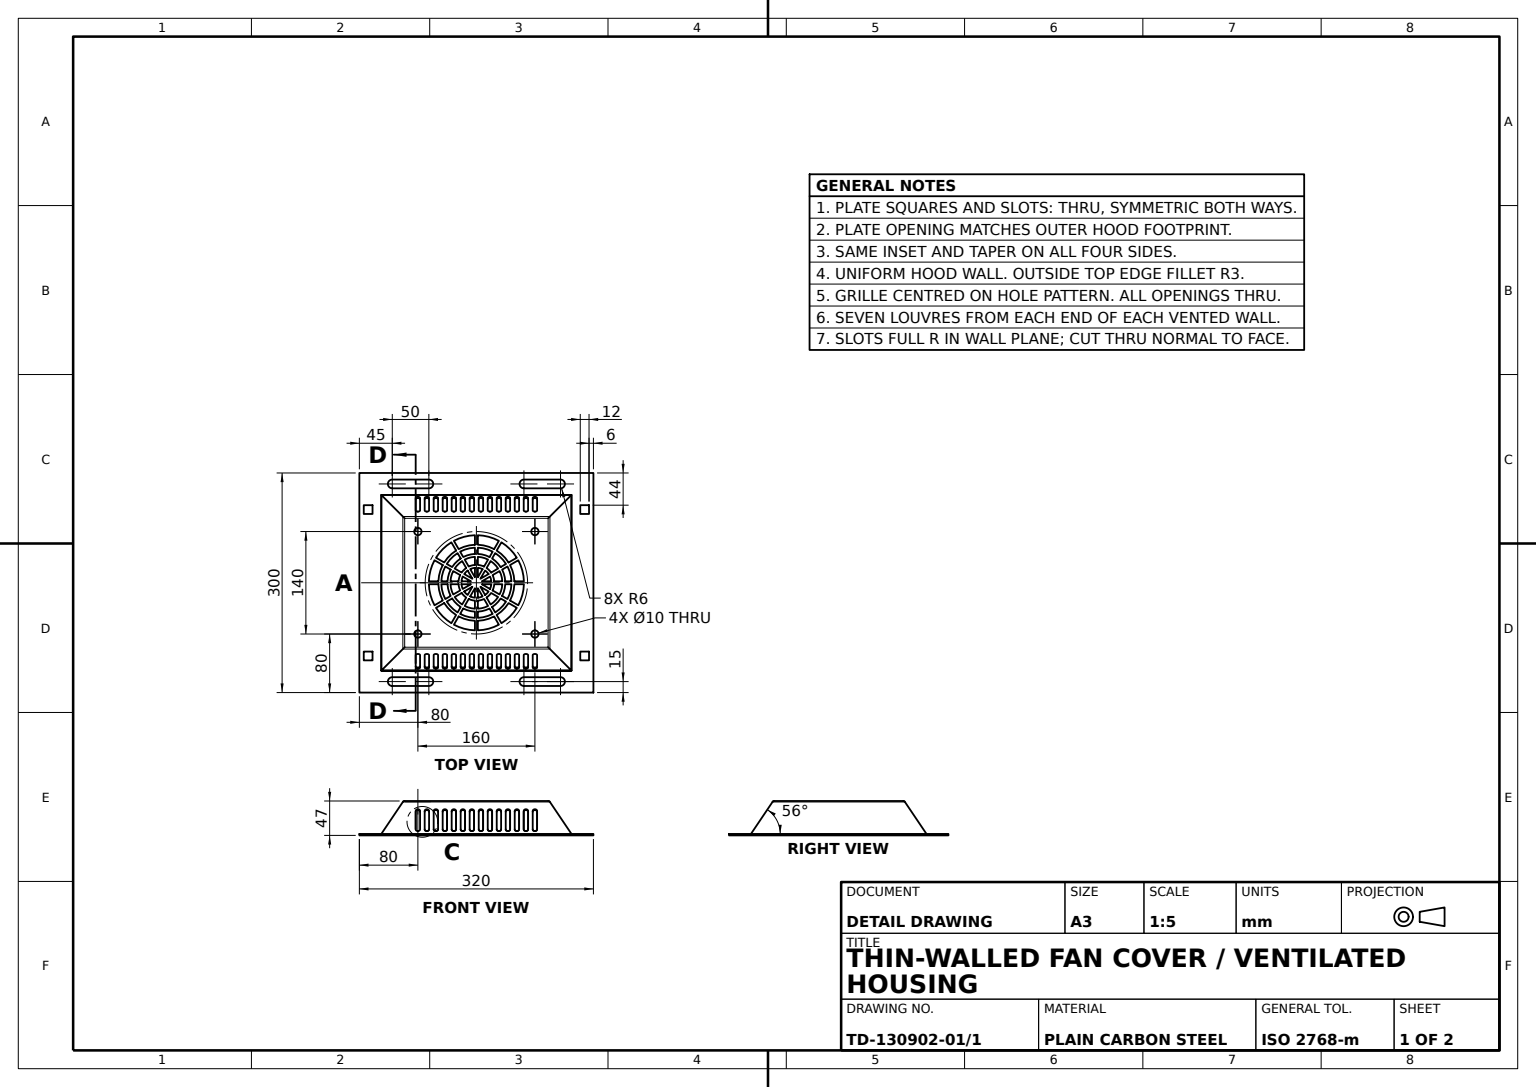
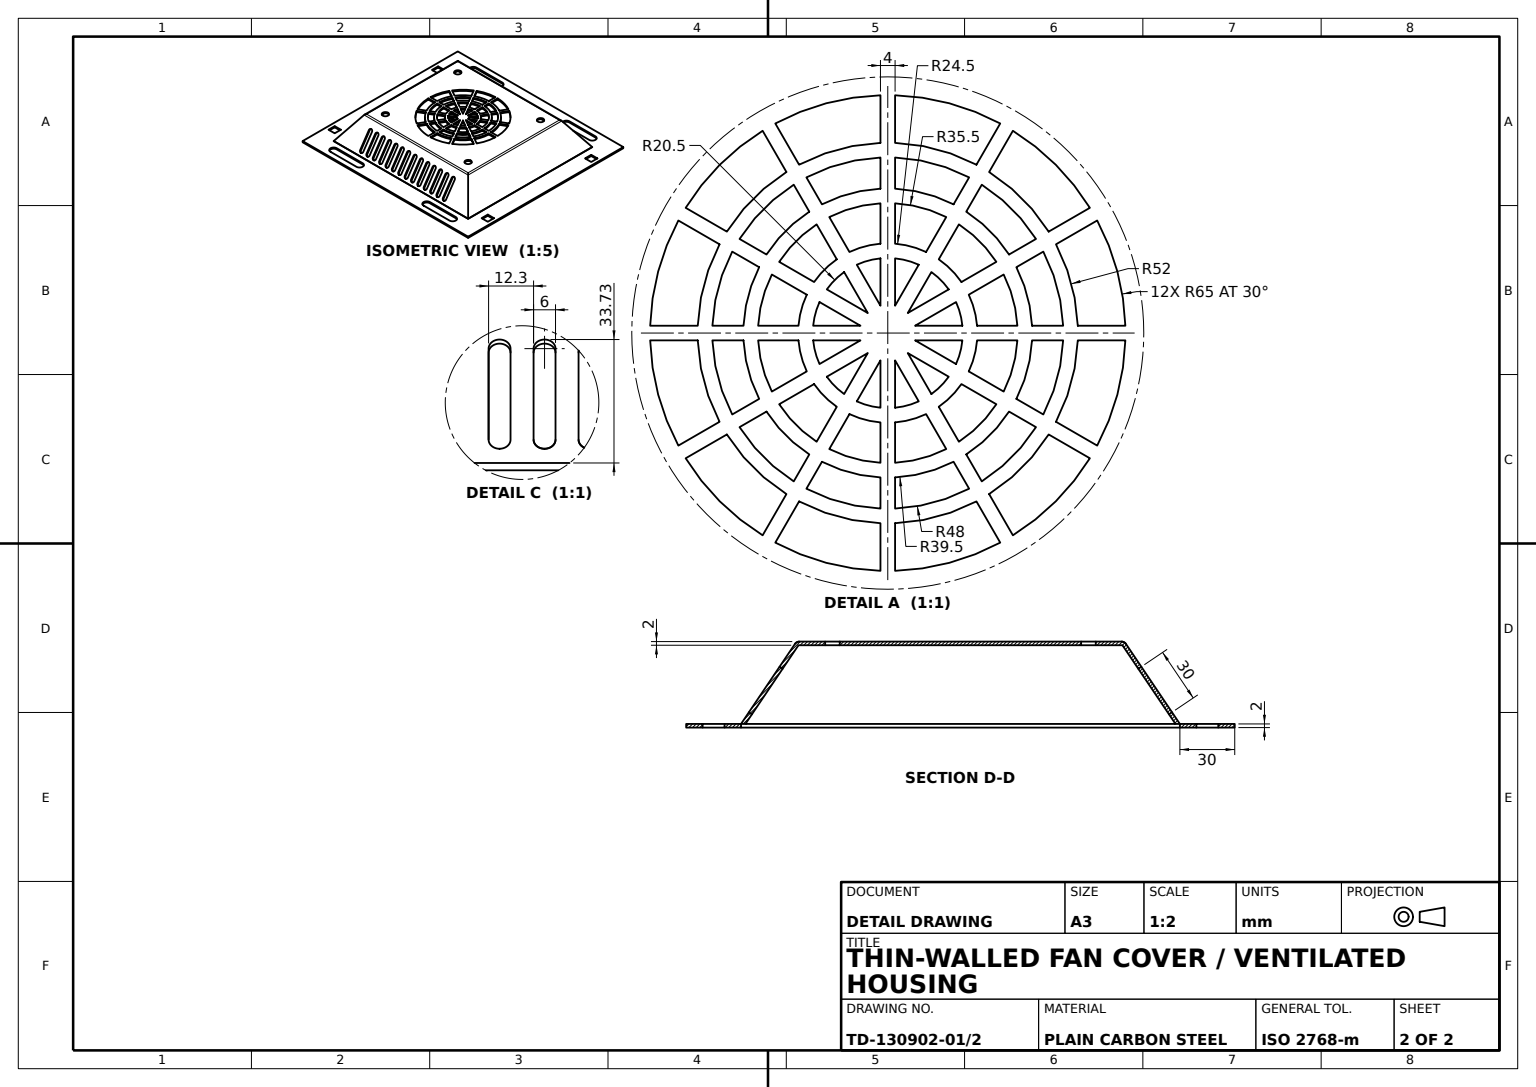
SolidWorks part; units mm, degrees
material "Plain Carbon Steel"
ref_plane "Front Plane" through (0, 0, 0) normal (0, 0, 1) x (1, 0, 0)
ref_plane "Top Plane" through (0, 0, 0) normal (0, 1, 0) x (1, 0, 0)
ref_plane "Right Plane" through (0, 0, 0) normal (1, 0, 0) x (0, 0, -1)
sketch "Base Plate Sketch" plane through (0, 0, 0) normal (0, 1, 0) x (1, 0, 0)
  line L1 (-160, -150) -> (160, -150)
  line L2 (-160, -150) -> (-160, 150)
  line L3 (-160, 150) -> (160, 150)
  line L4 (160, -150) -> (160, 150)
  line L5 (-160, -150) -> (160, 150) construction
  line L6 (-160, 150) -> (160, -150) construction
  point P0 (0, 0)
  dimension "D1" = 320
  dimension "D2" = 300
extrude "Base Plate 320x300x2" add sketch "Base Plate Sketch" along normal blind 2
sketch "Hood Footprint Sketch" plane through (0, 2, 0) normal (0, 1, 0) x (1, 0, 0)
  line L0 (-160, 150) -> (-160, -150) construction
  line L1 (-130, -120) -> (130, -120)
  line L2 (-130, -120) -> (-130, 120)
  line L3 (-130, 120) -> (130, 120)
  line L4 (130, -120) -> (130, 120)
  line L5 (-130, -120) -> (130, 120) construction
  line L6 (-130, 120) -> (130, -120) construction
  line L8 (-160, -150) -> (160, -150) construction
  point P0 (0, 0)
  dimension "D1" = 30
  dimension "D2" = 30
extrude "Tapered Hood H45" add sketch "Hood Footprint Sketch" along normal blind 45 draft 34
sketch "Hood Opening Sketch" plane through (0, 0, 0) normal (0, -1, 0) x (1, 0, 0)
  line L0 (-160, -150) -> (-160, 150) construction
  line L1 (-130, -120) -> (130, -120)
  line L2 (-130, -120) -> (-130, 120)
  line L3 (-130, 120) -> (130, 120)
  line L4 (130, -120) -> (130, 120)
  line L5 (-130, -120) -> (130, 120) construction
  line L6 (-130, 120) -> (130, -120) construction
  line L7 (160, -150) -> (-160, -150) construction
  point P0 (0, 0)
  dimension "D1" = 30
  dimension "D2" = 30
extrude "Hood Underside Opening" cut sketch "Hood Opening Sketch" against normal blind 2
shell "Hood Shell 2mm" thickness 2
sketch "Fan Grille Sketch" plane through (0, 47, 0) normal (0, 1, 0) x (1, 0, 0)
  line L0 (0, -69.2804) -> (0, 71.303) construction
  line L1 (2, -64.9692) -> (2, -51.9615)
  line L2 (-2, -64.9692) -> (-2, -51.9615)
  line L3 (-70.7733, 0) -> (72.5907, 0) construction
  line L4 (0, 0) -> (38.06, -65.9219) construction
  line L5 (2, -7.4641) -> (8.4691, -18.6688)
  line L6 (5.4641, -5.4641) -> (11.9332, -16.6688)
  line L7 (0, 0) -> (65.3908, -37.7534) construction
  line L8 (5.4641, -5.4641) -> (16.6688, -11.9332)
  line L9 (7.4641, -2) -> (18.6688, -8.4691)
  line L10 (0, 0) -> (68.8781, 39.7668) construction
  line L11 (7.4641, 2) -> (18.6688, 8.4691)
  line L12 (27.7128, -44) -> (34.2167, -55.265)
  line L13 (0, 0) -> (36.7024, 63.5704) construction
  line L14 (5.4641, 5.4641) -> (11.9332, 16.6688)
  line L15 (2, 7.4641) -> (8.4691, 18.6688)
  line L16 (0, 0) -> (-40.3307, 69.8548) construction
  line L17 (-47.9583, 2) -> (-39.4493, 2)
  line L18 (99.6471, -89.6471) -> (99.6471, 89.6471) construction
  line L19 (0, 0) -> (-67.6779, 39.0739) construction
  line L20 (7.4641, 2) -> (20.4022, 2)
  line L21 (-7.4641, 2) -> (-18.6688, 8.4691)
  line L22 (0, 0) -> (-64.8015, -37.4132) construction
  line L23 (0, 0) -> (-36.7564, -63.6639) construction
  line L24 (-27.7128, -44) -> (-34.2167, -55.265)
  line L25 (46, -24.2487) -> (57.265, -30.7526)
  line L26 (-5.4641, -5.4641) -> (-11.9332, -16.6688)
  line L27 (99.6471, 89.6471) -> (-99.6471, 89.6471) construction
  line L28 (-64.9692, -2) -> (-51.9615, -2)
  line L29 (-64.9692, 2) -> (-51.9615, 2)
  line L30 (-27.7128, 44) -> (-34.2167, 55.265)
  line L31 (-47.9583, -2) -> (-39.4493, -2)
  line L32 (-35.4436, 2) -> (-24.4182, 2)
  line L33 (-24.2487, 46) -> (-30.7526, 57.265)
  line L34 (-21.4567, 33.1641) -> (-25.7112, 40.5331)
  line L35 (-17.9926, 35.1641) -> (-22.2471, 42.5331)
  line L36 (-10.4771, 22.1468) -> (-15.9898, 31.6951)
  line L37 (-13.9412, 20.1468) -> (-19.4539, 29.6951)
  line L38 (-5.4641, 5.4641) -> (-11.9332, 16.6688)
  line L39 (-2, 7.4641) -> (-8.4691, 18.6688)
  line L40 (-2, 7.4641) -> (-2, 20.4022)
  line L41 (-46, 24.2487) -> (-57.265, 30.7526)
  line L43 (-35.4436, -2) -> (-24.4182, -2)
  line L45 (-44, 27.7128) -> (-55.265, 34.2167)
  line L46 (-35.1641, 17.9926) -> (-42.5331, 22.2471)
  line L47 (-33.1641, 21.4567) -> (-40.5331, 25.7112)
  line L48 (-22.1468, 10.4771) -> (-31.6951, 15.9898)
  line L49 (-20.1468, 13.9412) -> (-29.6951, 19.4539)
  line L50 (-5.4641, 5.4641) -> (-16.6688, 11.9332)
  line L52 (-20.4022, 2) -> (-7.4641, 2)
  line L53 (-20.4022, -2) -> (-7.4641, -2)
  line L54 (-46, -24.2487) -> (-57.265, -30.7526)
  line L57 (-44, -27.7128) -> (-55.265, -34.2167)
  line L58 (-35.1641, -17.9926) -> (-42.5331, -22.2471)
  line L59 (-33.1641, -21.4567) -> (-40.5331, -25.7112)
  line L60 (-20.1468, -13.9412) -> (-29.6951, -19.4539)
  line L61 (-22.1468, -10.4771) -> (-31.6951, -15.9898)
  line L62 (-5.4641, -5.4641) -> (-16.6688, -11.9332)
  line L63 (-7.4641, -2) -> (-18.6688, -8.4691)
  line L64 (7.4641, -2) -> (20.4022, -2)
  line L66 (44, -27.7128) -> (55.265, -34.2167)
  line L67 (-24.2487, -46) -> (-30.7526, -57.265)
  line L68 (-21.4567, -33.1641) -> (-25.7112, -40.5331)
  line L69 (-17.9926, -35.1641) -> (-22.2471, -42.5331)
  line L70 (-13.9412, -20.1468) -> (-19.4539, -29.6951)
  line L71 (-10.4771, -22.1468) -> (-15.9898, -31.6951)
  line L72 (-2, -47.9583) -> (-2, -39.4493)
  line L74 (2, -47.9583) -> (2, -39.4493)
  line L75 (-2, -35.4436) -> (-2, -24.4182)
  line L76 (2, -35.4436) -> (2, -24.4182)
  line L78 (5.4641, 5.4641) -> (16.6688, 11.9332)
  line L80 (24.2487, -46) -> (30.7526, -57.265)
  line L81 (21.4567, -33.1641) -> (25.7112, -40.5331)
  line L82 (17.9926, -35.1641) -> (22.2471, -42.5331)
  line L83 (13.9412, -20.1468) -> (19.4539, -29.6951)
  line L84 (10.4771, -22.1468) -> (15.9898, -31.6951)
  line L85 (-2, -20.4022) -> (-2, -7.4641)
  line L86 (2, -20.4022) -> (2, -7.4641)
  line L87 (-2, -7.4641) -> (-8.4691, -18.6688)
  line L88 (2, 7.4641) -> (2, 20.4022)
  line L89 (33.1641, -21.4567) -> (40.5331, -25.7112)
  line L90 (35.1641, -17.9926) -> (42.5331, -22.2471)
  line L91 (20.1468, -13.9412) -> (29.6951, -19.4539)
  line L92 (22.1468, -10.4771) -> (31.6951, -15.9898)
  line L93 (51.9615, -2) -> (64.9692, -2)
  line L96 (51.9615, 2) -> (64.9692, 2)
  line L97 (39.4493, -2) -> (47.9583, -2)
  line L98 (39.4493, 2) -> (47.9583, 2)
  line L99 (24.4182, 2) -> (35.4436, 2)
  line L100 (24.4182, -2) -> (35.4436, -2)
  line L101 (44, 27.7128) -> (55.265, 34.2167)
  line L102 (46, 24.2487) -> (57.265, 30.7526)
  line L103 (33.1641, 21.4567) -> (40.5331, 25.7112)
  line L104 (35.1641, 17.9926) -> (42.5331, 22.2471)
  line L105 (20.1468, 13.9412) -> (29.6951, 19.4539)
  line L106 (22.1468, 10.4771) -> (31.6951, 15.9898)
  line L107 (27.7128, 44) -> (34.2167, 55.265)
  line L108 (24.2487, 46) -> (30.7526, 57.265)
  line L109 (17.9926, 35.1641) -> (22.2471, 42.5331)
  line L110 (21.4567, 33.1641) -> (25.7112, 40.5331)
  line L111 (10.4771, 22.1468) -> (15.9898, 31.6951)
  line L112 (13.9412, 20.1468) -> (19.4539, 29.6951)
  line L113 (2, 51.9615) -> (2, 64.9692)
  line L114 (-2, 51.9615) -> (-2, 64.9692)
  line L115 (2, 39.4493) -> (2, 47.9583)
  line L116 (-2, 39.4493) -> (-2, 47.9583)
  line L117 (-2, 24.4182) -> (-2, 35.4436)
  line L118 (2, 24.4182) -> (2, 35.4436)
  arc A0 (-34.2167, 55.265) -> (-55.265, 34.2167) centre (0, 0) ccw
  circle A1 centre (0, 0) radius 50 construction
  circle A2 centre (0, 0) radius 37.5 construction
  circle A3 centre (0, 0) radius 22.5 construction
  arc A5 (-27.7128, 44) -> (-44, 27.7128) centre (0, 0) ccw
  arc A6 (-25.7112, 40.5331) -> (-40.5331, 25.7112) centre (0, 0) ccw
  arc A7 (-21.4567, 33.1641) -> (-33.1641, 21.4567) centre (0, 0) ccw
  arc A8 (-19.4539, 29.6951) -> (-29.6951, 19.4539) centre (0, 0) ccw
  arc A9 (-13.9412, 20.1468) -> (-20.1468, 13.9412) centre (0, 0) ccw
  arc A10 (-11.9332, 16.6688) -> (-16.6688, 11.9332) centre (0, 0) ccw
  arc A11 (-57.265, 30.7526) -> (-64.9692, 2) centre (0, 0) ccw
  circle A12 centre (0, 0) radius 52 construction
  circle A13 centre (0, 0) radius 48 construction
  circle A14 centre (0, 0) radius 39.5 construction
  circle A15 centre (0, 0) radius 35.5 construction
  circle A16 centre (0, 0) radius 24.5 construction
  circle A17 centre (0, 0) radius 20.5 construction
  arc A18 (-46, 24.2487) -> (-51.9615, 2) centre (0, 0) ccw
  arc A19 (-42.5331, 22.2471) -> (-47.9583, 2) centre (0, 0) ccw
  arc A20 (-35.1641, 17.9926) -> (-39.4493, 2) centre (0, 0) ccw
  arc A21 (-31.6951, 15.9898) -> (-35.4436, 2) centre (0, 0) ccw
  arc A22 (-22.1468, 10.4771) -> (-24.4182, 2) centre (0, 0) ccw
  arc A23 (-18.6688, 8.4691) -> (-20.4022, 2) centre (0, 0) ccw
  arc A24 (-64.9692, -2) -> (-57.265, -30.7526) centre (0, 0) ccw
  arc A25 (-51.9615, -2) -> (-46, -24.2487) centre (0, 0) ccw
  arc A26 (-47.9583, -2) -> (-42.5331, -22.2471) centre (0, 0) ccw
  arc A27 (-39.4493, -2) -> (-35.1641, -17.9926) centre (0, 0) ccw
  arc A28 (-35.4436, -2) -> (-31.6951, -15.9898) centre (0, 0) ccw
  arc A29 (-24.4182, -2) -> (-22.1468, -10.4771) centre (0, 0) ccw
  arc A30 (-20.4022, -2) -> (-18.6688, -8.4691) centre (0, 0) ccw
  arc A31 (-55.265, -34.2167) -> (-34.2167, -55.265) centre (0, 0) ccw
  arc A32 (-44, -27.7128) -> (-27.7128, -44) centre (0, 0) ccw
  arc A33 (-40.5331, -25.7112) -> (-25.7112, -40.5331) centre (0, 0) ccw
  arc A34 (-33.1641, -21.4567) -> (-21.4567, -33.1641) centre (0, 0) ccw
  arc A35 (-29.6951, -19.4539) -> (-19.4539, -29.6951) centre (0, 0) ccw
  arc A36 (-20.1468, -13.9412) -> (-13.9412, -20.1468) centre (0, 0) ccw
  arc A37 (-16.6688, -11.9332) -> (-11.9332, -16.6688) centre (0, 0) ccw
  arc A38 (-30.7526, -57.265) -> (-2, -64.9692) centre (0, 0) ccw
  arc A39 (-24.2487, -46) -> (-2, -51.9615) centre (0, 0) ccw
  arc A40 (-22.2471, -42.5331) -> (-2, -47.9583) centre (0, 0) ccw
  arc A41 (-17.9926, -35.1641) -> (-2, -39.4493) centre (0, 0) ccw
  arc A42 (-15.9898, -31.6951) -> (-2, -35.4436) centre (0, 0) ccw
  arc A43 (-10.4771, -22.1468) -> (-2, -24.4182) centre (0, 0) ccw
  arc A44 (-8.4691, -18.6688) -> (-2, -20.4022) centre (0, 0) ccw
  arc A45 (2, -64.9692) -> (30.7526, -57.265) centre (0, 0) ccw
  arc A46 (2, -51.9615) -> (24.2487, -46) centre (0, 0) ccw
  arc A47 (2, -47.9583) -> (22.2471, -42.5331) centre (0, 0) ccw
  arc A48 (2, -39.4493) -> (17.9926, -35.1641) centre (0, 0) ccw
  arc A49 (2, -35.4436) -> (15.9898, -31.6951) centre (0, 0) ccw
  arc A50 (2, -24.4182) -> (10.4771, -22.1468) centre (0, 0) ccw
  arc A51 (34.2167, -55.265) -> (55.265, -34.2167) centre (0, 0) ccw
  arc A52 (27.7128, -44) -> (44, -27.7128) centre (0, 0) ccw
  arc A53 (25.7112, -40.5331) -> (40.5331, -25.7112) centre (0, 0) ccw
  arc A54 (21.4567, -33.1641) -> (33.1641, -21.4567) centre (0, 0) ccw
  arc A55 (19.4539, -29.6951) -> (29.6951, -19.4539) centre (0, 0) ccw
  arc A56 (13.9412, -20.1468) -> (20.1468, -13.9412) centre (0, 0) ccw
  arc A57 (11.9332, -16.6688) -> (16.6688, -11.9332) centre (0, 0) ccw
  arc A58 (2, -20.4022) -> (8.4691, -18.6688) centre (0, 0) ccw
  arc A59 (57.265, -30.7526) -> (64.9692, -2) centre (0, 0) ccw
  arc A60 (46, -24.2487) -> (51.9615, -2) centre (0, 0) ccw
  arc A61 (42.5331, -22.2471) -> (47.9583, -2) centre (0, 0) ccw
  arc A62 (35.1641, -17.9926) -> (39.4493, -2) centre (0, 0) ccw
  arc A63 (31.6951, -15.9898) -> (35.4436, -2) centre (0, 0) ccw
  arc A64 (22.1468, -10.4771) -> (24.4182, -2) centre (0, 0) ccw
  arc A65 (18.6688, -8.4691) -> (20.4022, -2) centre (0, 0) ccw
  arc A66 (64.9692, 2) -> (57.265, 30.7526) centre (0, 0) ccw
  arc A67 (51.9615, 2) -> (46, 24.2487) centre (0, 0) ccw
  arc A68 (47.9583, 2) -> (42.5331, 22.2471) centre (0, 0) ccw
  arc A69 (39.4493, 2) -> (35.1641, 17.9926) centre (0, 0) ccw
  arc A70 (35.4436, 2) -> (31.6951, 15.9898) centre (0, 0) ccw
  arc A71 (24.4182, 2) -> (22.1468, 10.4771) centre (0, 0) ccw
  arc A72 (20.4022, 2) -> (18.6688, 8.4691) centre (0, 0) ccw
  arc A73 (55.265, 34.2167) -> (34.2167, 55.265) centre (0, 0) ccw
  arc A74 (44, 27.7128) -> (27.7128, 44) centre (0, 0) ccw
  arc A75 (40.5331, 25.7112) -> (25.7112, 40.5331) centre (0, 0) ccw
  arc A76 (33.1641, 21.4567) -> (21.4567, 33.1641) centre (0, 0) ccw
  arc A77 (29.6951, 19.4539) -> (19.4539, 29.6951) centre (0, 0) ccw
  arc A78 (20.1468, 13.9412) -> (13.9412, 20.1468) centre (0, 0) ccw
  arc A79 (16.6688, 11.9332) -> (11.9332, 16.6688) centre (0, 0) ccw
  arc A80 (30.7526, 57.265) -> (-30.7526, 57.265) centre (0, 0) ccw
  arc A81 (24.2487, 46) -> (2, 51.9615) centre (0, 0) ccw
  arc A82 (22.2471, 42.5331) -> (2, 47.9583) centre (0, 0) ccw
  arc A83 (17.9926, 35.1641) -> (2, 39.4493) centre (0, 0) ccw
  arc A84 (15.9898, 31.6951) -> (2, 35.4436) centre (0, 0) ccw
  arc A85 (10.4771, 22.1468) -> (2, 24.4182) centre (0, 0) ccw
  arc A86 (8.4691, 18.6688) -> (2, 20.4022) centre (0, 0) ccw
  arc A87 (-2, 51.9615) -> (-24.2487, 46) centre (0, 0) ccw
  arc A88 (-2, 47.9583) -> (-22.2471, 42.5331) centre (0, 0) ccw
  arc A89 (-2, 39.4493) -> (-17.9926, 35.1641) centre (0, 0) ccw
  arc A90 (-2, 35.4436) -> (-15.9898, 31.6951) centre (0, 0) ccw
  arc A91 (-2, 24.4182) -> (-10.4771, 22.1468) centre (0, 0) ccw
  arc A92 (-2, 20.4022) -> (-8.4691, 18.6688) centre (0, 0) ccw
  point P1 (52, 0)
  point P9 (39.5, 0)
  point P13 (24.5, 0)
  point P20 (2, -69.2804)
  point P21 (2, 71.303)
  point P22 (-2, -69.2804)
  point P23 (-2, 71.303)
  point P26 (-1.7321, -1)
  point P28 (36.328, -66.9219)
  point P29 (1.7321, 1)
  point P30 (39.7921, -64.9219)
  point P31 (-1, -1.7321)
  point P33 (64.3908, -39.4854)
  point P34 (1, 1.7321)
  point P35 (66.3908, -36.0213)
  point P36 (1, -1.7321)
  point P38 (69.8781, 38.0347)
  point P41 (1.7321, -1)
  point P43 (38.4344, 62.5704)
  point P44 (-1.7321, 1)
  point P45 (34.9703, 64.5704)
  point P46 (1.7321, 1)
  point P48 (-38.5986, 70.8548)
  point P49 (-1.7321, -1)
  point P50 (-42.0627, 68.8548)
  point P51 (1, 1.7321)
  point P53 (-66.6779, 40.8059)
  point P54 (-1, -1.7321)
  point P55 (-68.6779, 37.3418)
  point P56 (-1, 1.7321)
  point P59 (-65.8015, -35.6811)
  point P60 (1, -1.7321)
  point P61 (-63.8015, -39.1452)
  point P62 (-1.7321, 1)
  point P63 (-38.4884, -62.6639)
  point P64 (0, 0)
  point P65 (-35.0243, -64.6639)
  point P66 (-70.7733, -2)
  point P67 (72.5907, -2)
  point P68 (-70.7733, 2)
  point P69 (72.5907, 2)
  point P75 (48, 0)
  point P79 (35.5, 0)
  point P85 (20.5, 0)
  dimension "D2" = 100
  dimension "D3" = 75
  dimension "D4" = 45
  dimension "D5" = 65
  dimension "D6" = 52
  dimension "D7" = 48
  dimension "D8" = 39.5
  dimension "D9" = 35.5
  dimension "D10" = 24.5
  dimension "D11" = 20.5
  dimension "D12" = 34.6779
  dimension "D14" = 42.3821
  dimension "D15" = 44.3821
  dimension "D17" = 47.6856
  dimension "D18" = 53.6471
  dimension "D20" = 55.6471
  dimension "D21" = 57.114
  dimension "D23" = 59.114
  dimension "D24" = 64.483
  dimension "D26" = 65.4305
  dimension "D27" = 66.483
  dimension "D29" = 67.952
  dimension "D30" = 68.8946
  dimension "D33" = 69.952
  dimension "D34" = 71.9343
  dimension "D35" = 73.9359
  dimension "D36" = 75.3984
  dimension "D37" = 77.4
  dimension "D38" = 77.5003
  dimension "D39" = 78.1904
  dimension "D40" = 79.5003
  dimension "D41" = 80.1933
  dimension "D42" = 80.9783
  dimension "D43" = 81.6545
  dimension "D44" = 82.9783
  dimension "D45" = 83.6574
  dimension "D46" = 85.706
  dimension "D47" = 87.714
  dimension "D48" = 89.1701
  dimension "D49" = 91.1781
  dimension "D50" = 92.183
  dimension "D51" = 94.183
  dimension "D52" = 97.6471
  dimension "D53" = 105.1112
  dimension "D54" = 107.1112
  dimension "D55" = 24.6779
  dimension "D56" = 32.3821
  dimension "D57" = 82.183
  dimension "D58" = 84.183
  dimension "D59" = 95.1112
  dimension "D60" = 97.1112
  dimension "D13" = 30
  dimension "D16" = 30
  dimension "D19" = 30
  dimension "D22" = 30
  dimension "D25" = 30
  dimension "D28" = 30
  dimension "D31" = 30
  dimension "D32" = 30
extrude "Fan Grille Cut" cut sketch "Fan Grille Sketch" against normal blind 2 contours A5 L30 A0 L45 | A87 L114 A80 L33 | A81 L108 A80 L113 | A74 L101 A73 L107 | A67 L96 A66 L102 | A60 L25 A59 L93 | A52 L12 A51 L66 | A46 L1 A45 L80 | A39 L67 A38 L2 | A32 L57 A31 L24 | A25 L28 A24 L54 | A18 L41 A11 L29 | A20 L46 A19 L17 | A7 L34 A6 L47 | A89 L116 A88 L35 | A83 L109 A82 L115 | A76 L103 A75 L110 | A69 L98 A68 L104 | A62 L90 A61 L97 | A54 L81 A53 L89 | A48 L74 A47 L82 | A41 L69 A40 L72 | A34 L59 A33 L68 | A27 L31 A26 L58 | A43 L71 A42 L75 | A36 L60 A35 L70 | A29 L43 A28 L61 | A22 L48 A21 L32 | A9 L37 A8 L49 | A91 L117 A90 L36 | A85 L111 A84 L118 | A78 L105 A77 L112 | A71 L99 A70 L106 | A64 L92 A63 L100 | A56 L83 A55 L91 | A50 L76 A49 L84 | L15 A86 L88 | L78 A79 L14 | L20 A72 L11 | L9 A65 L64 | L6 A57 L8 | L86 A58 L5 | L87 A44 L85 | L62 A37 L26 | L53 A30 L63 | L21 A23 L52 | L38 A10 L50 | L40 A92 L39
fillet "Hood Edge Fillet R3" radius 3 4 edges at (0, 47, 89.6471) (99.6471, 47, 0) (0, 47, -89.6471) (-99.6471, 47, 0)
sketch "Louvre Slots Side A Sketch" plane through (0, 56.2564, 83.4036) normal (0, 0.5592, 0.829) x (1, 0, 0)
  line L0 (-80, -27.7604) -> (-80, -57.7604) construction
  line L1 (-77, -27.7604) -> (-77, -57.7604)
  line L2 (-83, -27.7604) -> (-83, -57.7604)
  line L3 (100.5391, -12.7604) -> (-100.5391, -12.7604) construction
  line L4 (80, -27.7604) -> (80, -57.7604) construction
  line L5 (83, -27.7604) -> (83, -57.7604)
  line L6 (77, -27.7604) -> (77, -57.7604)
  line L7 (67.7, -27.7604) -> (67.7, -57.7604) construction
  line L8 (70.7, -27.7604) -> (70.7, -57.7604)
  line L9 (64.7, -27.7604) -> (64.7, -57.7604)
  line L10 (55.4, -27.7604) -> (55.4, -57.7604) construction
  line L11 (58.4, -27.7604) -> (58.4, -57.7604)
  line L12 (52.4, -27.7604) -> (52.4, -57.7604)
  line L13 (43.1, -27.7604) -> (43.1, -57.7604) construction
  line L14 (46.1, -27.7604) -> (46.1, -57.7604)
  line L15 (40.1, -27.7604) -> (40.1, -57.7604)
  line L16 (30.8, -27.7604) -> (30.8, -57.7604) construction
  line L17 (33.8, -27.7604) -> (33.8, -57.7604)
  line L18 (27.8, -27.7604) -> (27.8, -57.7604)
  line L19 (18.5, -27.7604) -> (18.5, -57.7604) construction
  line L20 (21.5, -27.7604) -> (21.5, -57.7604)
  line L21 (15.5, -27.7604) -> (15.5, -57.7604)
  line L22 (6.2, -27.7604) -> (6.2, -57.7604) construction
  line L23 (9.2, -27.7604) -> (9.2, -57.7604)
  line L24 (3.2, -27.7604) -> (3.2, -57.7604)
  line L25 (-67.7, -27.7604) -> (-67.7, -57.7604) construction
  line L26 (-64.7, -27.7604) -> (-64.7, -57.7604)
  line L27 (-70.7, -27.7604) -> (-70.7, -57.7604)
  line L28 (-55.4, -27.7604) -> (-55.4, -57.7604) construction
  line L29 (-52.4, -27.7604) -> (-52.4, -57.7604)
  line L30 (-58.4, -27.7604) -> (-58.4, -57.7604)
  line L31 (-43.1, -27.7604) -> (-43.1, -57.7604) construction
  line L32 (-40.1, -27.7604) -> (-40.1, -57.7604)
  line L33 (-46.1, -27.7604) -> (-46.1, -57.7604)
  line L34 (-30.8, -27.7604) -> (-30.8, -57.7604) construction
  line L35 (-27.8, -27.7604) -> (-27.8, -57.7604)
  line L36 (-33.8, -27.7604) -> (-33.8, -57.7604)
  line L37 (-18.5, -27.7604) -> (-18.5, -57.7604) construction
  line L38 (-15.5, -27.7604) -> (-15.5, -57.7604)
  line L39 (-21.5, -27.7604) -> (-21.5, -57.7604)
  line L40 (-6.2, -27.7604) -> (-6.2, -57.7604) construction
  line L41 (-3.2, -27.7604) -> (-3.2, -57.7604)
  line L42 (-9.2, -27.7604) -> (-9.2, -57.7604)
  arc A0 (-77, -27.7604) -> (-83, -27.7604) centre (-80, -27.7604) ccw
  arc A1 (-83, -57.7604) -> (-77, -57.7604) centre (-80, -57.7604) ccw
  arc A2 (83, -27.7604) -> (77, -27.7604) centre (80, -27.7604) ccw
  arc A3 (77, -57.7604) -> (83, -57.7604) centre (80, -57.7604) ccw
  arc A4 (70.7, -27.7604) -> (64.7, -27.7604) centre (67.7, -27.7604) ccw
  arc A5 (64.7, -57.7604) -> (70.7, -57.7604) centre (67.7, -57.7604) ccw
  arc A6 (58.4, -27.7604) -> (52.4, -27.7604) centre (55.4, -27.7604) ccw
  arc A7 (52.4, -57.7604) -> (58.4, -57.7604) centre (55.4, -57.7604) ccw
  arc A8 (46.1, -27.7604) -> (40.1, -27.7604) centre (43.1, -27.7604) ccw
  arc A9 (40.1, -57.7604) -> (46.1, -57.7604) centre (43.1, -57.7604) ccw
  arc A10 (33.8, -27.7604) -> (27.8, -27.7604) centre (30.8, -27.7604) ccw
  arc A11 (27.8, -57.7604) -> (33.8, -57.7604) centre (30.8, -57.7604) ccw
  arc A12 (21.5, -27.7604) -> (15.5, -27.7604) centre (18.5, -27.7604) ccw
  arc A13 (15.5, -57.7604) -> (21.5, -57.7604) centre (18.5, -57.7604) ccw
  arc A14 (9.2, -27.7604) -> (3.2, -27.7604) centre (6.2, -27.7604) ccw
  arc A15 (3.2, -57.7604) -> (9.2, -57.7604) centre (6.2, -57.7604) ccw
  arc A16 (-64.7, -27.7604) -> (-70.7, -27.7604) centre (-67.7, -27.7604) ccw
  arc A17 (-70.7, -57.7604) -> (-64.7, -57.7604) centre (-67.7, -57.7604) ccw
  arc A18 (-52.4, -27.7604) -> (-58.4, -27.7604) centre (-55.4, -27.7604) ccw
  arc A19 (-58.4, -57.7604) -> (-52.4, -57.7604) centre (-55.4, -57.7604) ccw
  arc A20 (-40.1, -27.7604) -> (-46.1, -27.7604) centre (-43.1, -27.7604) ccw
  arc A21 (-46.1, -57.7604) -> (-40.1, -57.7604) centre (-43.1, -57.7604) ccw
  arc A22 (-27.8, -27.7604) -> (-33.8, -27.7604) centre (-30.8, -27.7604) ccw
  arc A23 (-33.8, -57.7604) -> (-27.8, -57.7604) centre (-30.8, -57.7604) ccw
  arc A24 (-15.5, -27.7604) -> (-21.5, -27.7604) centre (-18.5, -27.7604) ccw
  arc A25 (-21.5, -57.7604) -> (-15.5, -57.7604) centre (-18.5, -57.7604) ccw
  arc A26 (-3.2, -27.7604) -> (-9.2, -27.7604) centre (-6.2, -27.7604) ccw
  arc A27 (-9.2, -57.7604) -> (-3.2, -57.7604) centre (-6.2, -57.7604) ccw
  point P2 (-80, -42.7604)
  point P12 (80, -42.7604)
  point P17 (67.7, -42.7604)
  point P24 (55.4, -42.7604)
  point P31 (43.1, -42.7604)
  point P38 (30.8, -42.7604)
  point P45 (18.5, -42.7604)
  point P52 (6.2, -42.7604)
  point P59 (-67.7, -42.7604)
  point P66 (-55.4, -42.7604)
  point P73 (-43.1, -42.7604)
  point P80 (-30.8, -42.7604)
  point P87 (-18.5, -42.7604)
  point P94 (-6.2, -42.7604)
  dimension "D3" = 3
  dimension "D1" = 15
  dimension "D2" = 30
  dimension "D4" = 80
  dimension "D5" = 80
  dimension "D6" = 12.3
  dimension "D7" = 12.3
  dimension "D8" = 12.3
  dimension "D9" = 12.3
  dimension "D10" = 12.3
  dimension "D11" = 12.3
  dimension "D12" = 12.3
  dimension "D13" = 12.3
  dimension "D14" = 12.3
  dimension "D15" = 12.3
  dimension "D16" = 12.3
  dimension "D17" = 12.3
extrude "Louvre Slots Side A" cut sketch "Louvre Slots Side A Sketch" against normal blind 2
sketch "Louvre Slots Side B Sketch" plane through (0, 56.2564, -83.4036) normal (0, 0.5592, -0.829) x (-1, 0, 0)
  line L0 (-80, -27.7604) -> (-80, -57.7604) construction
  line L1 (-77, -27.7604) -> (-77, -57.7604)
  line L2 (-83, -27.7604) -> (-83, -57.7604)
  line L3 (80, -27.7604) -> (80, -57.7604) construction
  line L4 (83, -27.7604) -> (83, -57.7604)
  line L5 (77, -27.7604) -> (77, -57.7604)
  line L6 (100.5391, -12.7604) -> (-100.5391, -12.7604) construction
  line L7 (67.7, -27.7604) -> (67.7, -57.7604) construction
  line L8 (70.7, -27.7604) -> (70.7, -57.7604)
  line L9 (64.7, -27.7604) -> (64.7, -57.7604)
  line L10 (55.4, -27.7604) -> (55.4, -57.7604) construction
  line L11 (58.4, -27.7604) -> (58.4, -57.7604)
  line L12 (52.4, -27.7604) -> (52.4, -57.7604)
  line L13 (43.1, -27.7604) -> (43.1, -57.7604) construction
  line L14 (46.1, -27.7604) -> (46.1, -57.7604)
  line L15 (40.1, -27.7604) -> (40.1, -57.7604)
  line L16 (30.8, -27.7604) -> (30.8, -57.7604) construction
  line L17 (33.8, -27.7604) -> (33.8, -57.7604)
  line L18 (27.8, -27.7604) -> (27.8, -57.7604)
  line L19 (18.5, -27.7604) -> (18.5, -57.7604) construction
  line L20 (21.5, -27.7604) -> (21.5, -57.7604)
  line L21 (15.5, -27.7604) -> (15.5, -57.7604)
  line L22 (6.2, -27.7604) -> (6.2, -57.7604) construction
  line L23 (9.2, -27.7604) -> (9.2, -57.7604)
  line L24 (3.2, -27.7604) -> (3.2, -57.7604)
  line L25 (-67.7, -27.7604) -> (-67.7, -57.7604) construction
  line L26 (-64.7, -27.7604) -> (-64.7, -57.7604)
  line L27 (-70.7, -27.7604) -> (-70.7, -57.7604)
  line L28 (-55.4, -27.7604) -> (-55.4, -57.7604) construction
  line L29 (-52.4, -27.7604) -> (-52.4, -57.7604)
  line L30 (-58.4, -27.7604) -> (-58.4, -57.7604)
  line L31 (-43.1, -27.7604) -> (-43.1, -57.7604) construction
  line L32 (-40.1, -27.7604) -> (-40.1, -57.7604)
  line L33 (-46.1, -27.7604) -> (-46.1, -57.7604)
  line L34 (-30.8, -27.7604) -> (-30.8, -57.7604) construction
  line L35 (-27.8, -27.7604) -> (-27.8, -57.7604)
  line L36 (-33.8, -27.7604) -> (-33.8, -57.7604)
  line L37 (-18.5, -27.7604) -> (-18.5, -57.7604) construction
  line L38 (-15.5, -27.7604) -> (-15.5, -57.7604)
  line L39 (-21.5, -27.7604) -> (-21.5, -57.7604)
  line L40 (-6.2, -27.7604) -> (-6.2, -57.7604) construction
  line L41 (-3.2, -27.7604) -> (-3.2, -57.7604)
  line L42 (-9.2, -27.7604) -> (-9.2, -57.7604)
  arc A0 (-77, -27.7604) -> (-83, -27.7604) centre (-80, -27.7604) ccw
  arc A1 (-83, -57.7604) -> (-77, -57.7604) centre (-80, -57.7604) ccw
  arc A2 (83, -27.7604) -> (77, -27.7604) centre (80, -27.7604) ccw
  arc A3 (77, -57.7604) -> (83, -57.7604) centre (80, -57.7604) ccw
  arc A4 (70.7, -27.7604) -> (64.7, -27.7604) centre (67.7, -27.7604) ccw
  arc A5 (64.7, -57.7604) -> (70.7, -57.7604) centre (67.7, -57.7604) ccw
  arc A6 (58.4, -27.7604) -> (52.4, -27.7604) centre (55.4, -27.7604) ccw
  arc A7 (52.4, -57.7604) -> (58.4, -57.7604) centre (55.4, -57.7604) ccw
  arc A8 (46.1, -27.7604) -> (40.1, -27.7604) centre (43.1, -27.7604) ccw
  arc A9 (40.1, -57.7604) -> (46.1, -57.7604) centre (43.1, -57.7604) ccw
  arc A10 (33.8, -27.7604) -> (27.8, -27.7604) centre (30.8, -27.7604) ccw
  arc A11 (27.8, -57.7604) -> (33.8, -57.7604) centre (30.8, -57.7604) ccw
  arc A12 (21.5, -27.7604) -> (15.5, -27.7604) centre (18.5, -27.7604) ccw
  arc A13 (15.5, -57.7604) -> (21.5, -57.7604) centre (18.5, -57.7604) ccw
  arc A14 (9.2, -27.7604) -> (3.2, -27.7604) centre (6.2, -27.7604) ccw
  arc A15 (3.2, -57.7604) -> (9.2, -57.7604) centre (6.2, -57.7604) ccw
  arc A16 (-64.7, -27.7604) -> (-70.7, -27.7604) centre (-67.7, -27.7604) ccw
  arc A17 (-70.7, -57.7604) -> (-64.7, -57.7604) centre (-67.7, -57.7604) ccw
  arc A18 (-52.4, -27.7604) -> (-58.4, -27.7604) centre (-55.4, -27.7604) ccw
  arc A19 (-58.4, -57.7604) -> (-52.4, -57.7604) centre (-55.4, -57.7604) ccw
  arc A20 (-40.1, -27.7604) -> (-46.1, -27.7604) centre (-43.1, -27.7604) ccw
  arc A21 (-46.1, -57.7604) -> (-40.1, -57.7604) centre (-43.1, -57.7604) ccw
  arc A22 (-27.8, -27.7604) -> (-33.8, -27.7604) centre (-30.8, -27.7604) ccw
  arc A23 (-33.8, -57.7604) -> (-27.8, -57.7604) centre (-30.8, -57.7604) ccw
  arc A24 (-15.5, -27.7604) -> (-21.5, -27.7604) centre (-18.5, -27.7604) ccw
  arc A25 (-21.5, -57.7604) -> (-15.5, -57.7604) centre (-18.5, -57.7604) ccw
  arc A26 (-3.2, -27.7604) -> (-9.2, -27.7604) centre (-6.2, -27.7604) ccw
  arc A27 (-9.2, -57.7604) -> (-3.2, -57.7604) centre (-6.2, -57.7604) ccw
  point P2 (-80, -42.7604)
  point P7 (80, -42.7604)
  point P17 (67.7, -42.7604)
  point P24 (55.4, -42.7604)
  point P31 (43.1, -42.7604)
  point P38 (30.8, -42.7604)
  point P45 (18.5, -42.7604)
  point P52 (6.2, -42.7604)
  point P59 (-67.7, -42.7604)
  point P66 (-55.4, -42.7604)
  point P73 (-43.1, -42.7604)
  point P80 (-30.8, -42.7604)
  point P87 (-18.5, -42.7604)
  point P94 (-6.2, -42.7604)
  dimension "D3" = 3
  dimension "D1" = 15
  dimension "D2" = 30
  dimension "D4" = 80
  dimension "D5" = 80
  dimension "D6" = 12.3
  dimension "D7" = 12.3
  dimension "D8" = 12.3
  dimension "D9" = 12.3
  dimension "D10" = 12.3
  dimension "D11" = 12.3
  dimension "D12" = 12.3
  dimension "D13" = 12.3
  dimension "D14" = 12.3
  dimension "D15" = 12.3
  dimension "D16" = 12.3
  dimension "D17" = 12.3
extrude "Louvre Slots Side B" cut sketch "Louvre Slots Side B Sketch" against normal blind 2
sketch "Plate Mounting Slots Sketch" plane through (0, 2, 0) normal (0, 1, 0) x (1, 0, 0)
  line L0 (-115, -135) -> (-65, -135) construction
  line L1 (-115, -129) -> (-65, -129)
  line L2 (-115, -141) -> (-65, -141)
  line L3 (65, -135) -> (115, -135) construction
  line L4 (65, -129) -> (115, -129)
  line L5 (65, -141) -> (115, -141)
  line L6 (-115, 135) -> (-65, 135) construction
  line L7 (-115, 141) -> (-65, 141)
  line L8 (-115, 129) -> (-65, 129)
  line L9 (65, 135) -> (115, 135) construction
  line L10 (65, 141) -> (115, 141)
  line L11 (65, 129) -> (115, 129)
  line L12 (-160, 150) -> (-160, -150) construction
  line L13 (160, 150) -> (-160, 150) construction
  line L14 (160, -150) -> (160, 150) construction
  line L15 (-160, -150) -> (160, -150) construction
  line L17 (142, 94) -> (154, 94)
  line L18 (142, 94) -> (142, 106)
  line L19 (142, 106) -> (154, 106)
  line L20 (154, 94) -> (154, 106)
  line L21 (142, 94) -> (154, 106) construction
  line L22 (142, 106) -> (154, 94) construction
  line L23 (142, -106) -> (154, -106)
  line L24 (142, -106) -> (142, -94)
  line L25 (142, -94) -> (154, -94)
  line L26 (154, -106) -> (154, -94)
  line L27 (142, -106) -> (154, -94) construction
  line L28 (142, -94) -> (154, -106) construction
  line L29 (-154, -106) -> (-142, -106)
  line L30 (-154, -106) -> (-154, -94)
  line L31 (-154, -94) -> (-142, -94)
  line L32 (-142, -106) -> (-142, -94)
  line L33 (-154, -106) -> (-142, -94) construction
  line L34 (-154, -94) -> (-142, -106) construction
  line L35 (-154, 106) -> (-142, 106)
  line L36 (-154, 106) -> (-154, 94)
  line L37 (-154, 94) -> (-142, 94)
  line L38 (-142, 106) -> (-142, 94)
  line L39 (-154, 106) -> (-142, 94) construction
  line L40 (-154, 94) -> (-142, 106) construction
  arc A0 (-115, -129) -> (-115, -141) centre (-115, -135) ccw
  arc A1 (-65, -141) -> (-65, -129) centre (-65, -135) ccw
  arc A2 (65, -129) -> (65, -141) centre (65, -135) ccw
  arc A3 (115, -141) -> (115, -129) centre (115, -135) ccw
  arc A4 (-115, 141) -> (-115, 129) centre (-115, 135) ccw
  arc A5 (-65, 129) -> (-65, 141) centre (-65, 135) ccw
  arc A6 (65, 141) -> (65, 129) centre (65, 135) ccw
  arc A7 (115, 129) -> (115, 141) centre (115, 135) ccw
  point P2 (-90, -135)
  point P7 (90, -135)
  point P14 (-90, 135)
  point P21 (90, 135)
  point P36 (148, -100)
  point P38 (148, 100)
  point P46 (-148, -100)
  point P51 (-148, 100)
  dimension "D3" = 6
  dimension "D1" = 50
  dimension "D2" = 45
  dimension "D4" = 15
  dimension "D5" = 45
  dimension "D6" = 15
  dimension "D7" = 12
  dimension "D8" = 12
  dimension "D9" = 12
  dimension "D10" = 50
  dimension "D11" = 12
  dimension "D12" = 50
extrude "Plate Mounting Slots and Holes" cut sketch "Plate Mounting Slots Sketch" against normal blind 2
sketch "Hood Top Holes Sketch" plane through (0, 47, 0) normal (0, 1, 0) x (1, 0, 0)
  line L0 (0, 0) -> (0, 13.0665) construction
  line L1 (0, 0) -> (17.1483, 0) construction
  circle A0 centre (-80, 70) radius 5
  circle A1 centre (80, 70) radius 5
  circle A2 centre (80, -70) radius 5
  circle A3 centre (-80, -70) radius 5
  dimension "D1" = 10
  dimension "D2" = 160
  dimension "D3" = 140
extrude "Hood Top Fixing Holes" cut sketch "Hood Top Holes Sketch" against normal blind 2
